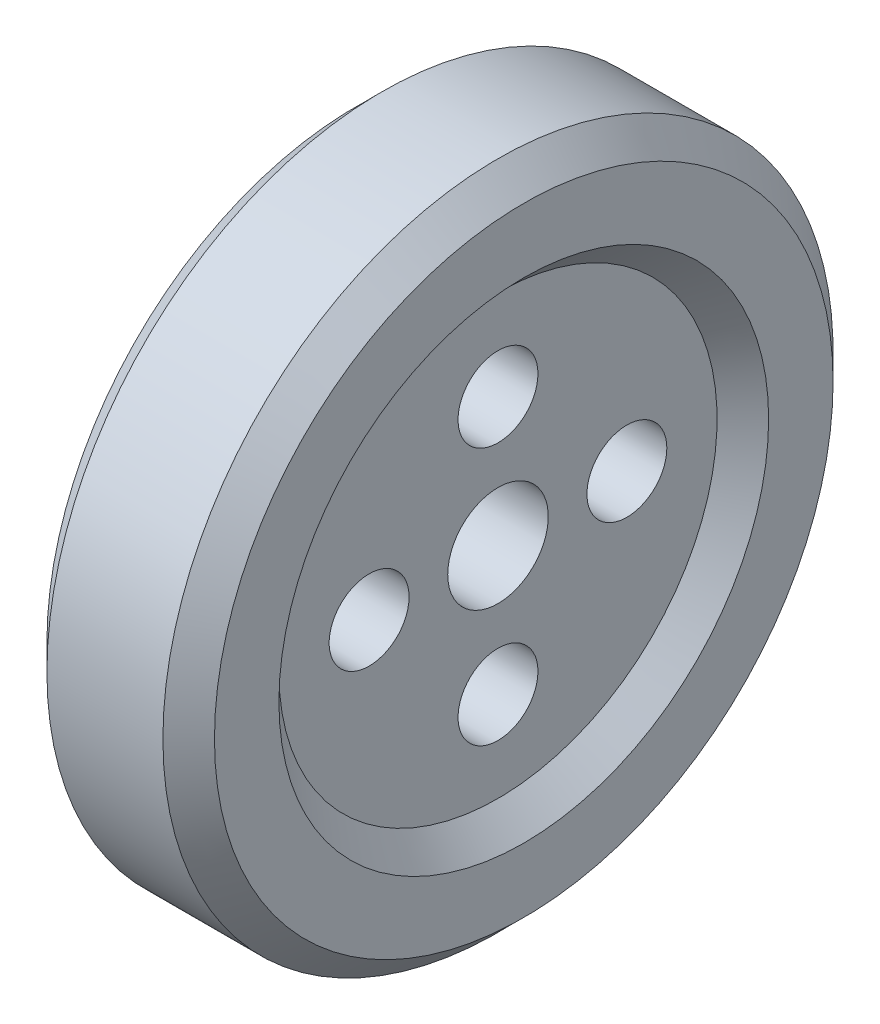
ISO-10303-21;
HEADER;
FILE_DESCRIPTION(('STEP AP214'),'2;1');
FILE_NAME('part.step','',(''),(''),'','','');
FILE_SCHEMA(('AUTOMOTIVE_DESIGN { 1 0 10303 214 1 1 1 1 }'));
ENDSEC;
DATA;
#1=APPLICATION_CONTEXT('core data for automotive mechanical design processes');
#2=APPLICATION_PROTOCOL_DEFINITION('international standard','automotive_design',2000,#1);
#3=PRODUCT_CONTEXT('',#1,'mechanical');
#4=PRODUCT('Part','Part','',(#3));
#5=PRODUCT_RELATED_PRODUCT_CATEGORY('part','',(#4));
#6=PRODUCT_DEFINITION_FORMATION('','',#4);
#7=PRODUCT_DEFINITION_CONTEXT('part definition',#1,'design');
#8=PRODUCT_DEFINITION('design','',#6,#7);
#9=PRODUCT_DEFINITION_SHAPE('','',#8);
#10=(LENGTH_UNIT() NAMED_UNIT(*) SI_UNIT(.MILLI.,.METRE.));
#11=(NAMED_UNIT(*) PLANE_ANGLE_UNIT() SI_UNIT($,.RADIAN.));
#12=(NAMED_UNIT(*) SI_UNIT($,.STERADIAN.) SOLID_ANGLE_UNIT());
#13=UNCERTAINTY_MEASURE_WITH_UNIT(LENGTH_MEASURE(1.E-05),#10,'distance_accuracy_value','');
#14=(GEOMETRIC_REPRESENTATION_CONTEXT(3) GLOBAL_UNCERTAINTY_ASSIGNED_CONTEXT((#13)) GLOBAL_UNIT_ASSIGNED_CONTEXT((#10,
#11,#12)) REPRESENTATION_CONTEXT('',''));
#15=CARTESIAN_POINT('',(0.,0.,0.));
#16=DIRECTION('',(0.,0.,1.));
#17=DIRECTION('',(1.,0.,0.));
#18=AXIS2_PLACEMENT_3D('',#15,#16,#17);
#19=CARTESIAN_POINT('',(-186.115918114073,0.,0.));
#20=DIRECTION('',(-1.,0.,0.));
#21=DIRECTION('',(0.,0.,1.));
#22=AXIS2_PLACEMENT_3D('',#19,#20,#21);
#23=CYLINDRICAL_SURFACE('',#22,260.);
#24=CARTESIAN_POINT('',(-45.,0.,0.));
#25=DIRECTION('',(-1.,0.,0.));
#26=DIRECTION('',(0.,0.,1.));
#27=AXIS2_PLACEMENT_3D('',#24,#25,#26);
#28=CIRCLE('',#27,260.);
#29=CARTESIAN_POINT('',(-45.,0.,260.));
#30=VERTEX_POINT('',#29);
#31=EDGE_CURVE('E10',#30,#30,#28,.T.);
#32=ORIENTED_EDGE('',*,*,#31,.F.);
#33=EDGE_LOOP('',(#32));
#34=FACE_BOUND('',#33,.T.);
#35=CARTESIAN_POINT('',(44.9999999999999,0.,0.));
#36=DIRECTION('',(-1.,0.,0.));
#37=DIRECTION('',(0.,0.,1.));
#38=AXIS2_PLACEMENT_3D('',#35,#36,#37);
#39=CIRCLE('',#38,260.);
#40=CARTESIAN_POINT('',(44.9999999999999,0.,260.));
#41=VERTEX_POINT('',#40);
#42=EDGE_CURVE('E72',#41,#41,#39,.T.);
#43=ORIENTED_EDGE('',*,*,#42,.T.);
#44=EDGE_LOOP('',(#43));
#45=FACE_BOUND('',#44,.T.);
#46=ADVANCED_FACE('F40',(#34,#45),#23,.T.);
#47=CARTESIAN_POINT('',(-45.,0.,0.));
#48=DIRECTION('',(1.,0.,0.));
#49=DIRECTION('',(0.,0.,-1.));
#50=AXIS2_PLACEMENT_3D('',#47,#48,#49);
#51=CONICAL_SURFACE('',#50,260.,0.785398163397452);
#52=CARTESIAN_POINT('',(-64.9999999999999,0.,0.));
#53=DIRECTION('',(-1.,0.,0.));
#54=DIRECTION('',(0.,0.,1.));
#55=AXIS2_PLACEMENT_3D('',#52,#53,#54);
#56=CIRCLE('',#55,240.);
#57=CARTESIAN_POINT('',(-64.9999999999999,0.,240.));
#58=VERTEX_POINT('',#57);
#59=EDGE_CURVE('E43',#58,#58,#56,.T.);
#60=ORIENTED_EDGE('',*,*,#59,.F.);
#61=EDGE_LOOP('',(#60));
#62=FACE_BOUND('',#61,.T.);
#63=ORIENTED_EDGE('',*,*,#31,.T.);
#64=EDGE_LOOP('',(#63));
#65=FACE_BOUND('',#64,.T.);
#66=ADVANCED_FACE('F136',(#62,#65),#51,.T.);
#67=CARTESIAN_POINT('',(-64.9999999999999,240.,0.));
#68=DIRECTION('',(1.,0.,0.));
#69=DIRECTION('',(0.,0.,-1.));
#70=AXIS2_PLACEMENT_3D('',#67,#68,#69);
#71=PLANE('',#70);
#72=CARTESIAN_POINT('',(-65.,0.,0.));
#73=DIRECTION('',(-1.,0.,0.));
#74=DIRECTION('',(0.,0.,1.));
#75=AXIS2_PLACEMENT_3D('',#72,#73,#74);
#76=CIRCLE('',#75,190.);
#77=CARTESIAN_POINT('',(-65.,0.,190.));
#78=VERTEX_POINT('',#77);
#79=EDGE_CURVE('E50',#78,#78,#76,.T.);
#80=ORIENTED_EDGE('',*,*,#79,.F.);
#81=EDGE_LOOP('',(#80));
#82=FACE_BOUND('',#81,.T.);
#83=ORIENTED_EDGE('',*,*,#59,.T.);
#84=EDGE_LOOP('',(#83));
#85=FACE_BOUND('',#84,.T.);
#86=ADVANCED_FACE('F135',(#82,#85),#71,.F.);
#87=CARTESIAN_POINT('',(-65.,0.,0.));
#88=DIRECTION('',(-1.,0.,0.));
#89=DIRECTION('',(0.,0.,1.));
#90=AXIS2_PLACEMENT_3D('',#87,#88,#89);
#91=CONICAL_SURFACE('',#90,190.,0.785398163397448);
#92=CARTESIAN_POINT('',(-45.,0.,0.));
#93=DIRECTION('',(-1.,0.,0.));
#94=DIRECTION('',(0.,0.,1.));
#95=AXIS2_PLACEMENT_3D('',#92,#93,#94);
#96=CIRCLE('',#95,170.);
#97=CARTESIAN_POINT('',(-45.,0.,170.));
#98=VERTEX_POINT('',#97);
#99=EDGE_CURVE('E51',#98,#98,#96,.T.);
#100=ORIENTED_EDGE('',*,*,#99,.F.);
#101=EDGE_LOOP('',(#100));
#102=FACE_BOUND('',#101,.T.);
#103=ORIENTED_EDGE('',*,*,#79,.T.);
#104=EDGE_LOOP('',(#103));
#105=FACE_BOUND('',#104,.T.);
#106=ADVANCED_FACE('F127',(#102,#105),#91,.F.);
#107=CARTESIAN_POINT('',(-45.,170.,0.));
#108=DIRECTION('',(1.,0.,0.));
#109=DIRECTION('',(0.,0.,-1.));
#110=AXIS2_PLACEMENT_3D('',#107,#108,#109);
#111=PLANE('',#110);
#112=CARTESIAN_POINT('',(-45.,100.,0.));
#113=DIRECTION('',(1.,0.,0.));
#114=DIRECTION('',(0.,0.,-1.));
#115=AXIS2_PLACEMENT_3D('',#112,#113,#114);
#116=CIRCLE('',#115,31.);
#117=CARTESIAN_POINT('',(-45.,100.,-31.));
#118=VERTEX_POINT('',#117);
#119=EDGE_CURVE('E74',#118,#118,#116,.F.);
#120=ORIENTED_EDGE('',*,*,#119,.F.);
#121=EDGE_LOOP('',(#120));
#122=FACE_BOUND('',#121,.T.);
#123=CARTESIAN_POINT('',(-45.,0.,-100.));
#124=DIRECTION('',(1.,0.,0.));
#125=DIRECTION('',(0.,0.,-1.));
#126=AXIS2_PLACEMENT_3D('',#123,#124,#125);
#127=CIRCLE('',#126,31.0000000000003);
#128=CARTESIAN_POINT('',(-45.,0.,-131.));
#129=VERTEX_POINT('',#128);
#130=EDGE_CURVE('E86',#129,#129,#127,.F.);
#131=ORIENTED_EDGE('',*,*,#130,.F.);
#132=EDGE_LOOP('',(#131));
#133=FACE_BOUND('',#132,.T.);
#134=CARTESIAN_POINT('',(-45.,-100.,0.));
#135=DIRECTION('',(1.,0.,0.));
#136=DIRECTION('',(0.,0.,-1.));
#137=AXIS2_PLACEMENT_3D('',#134,#135,#136);
#138=CIRCLE('',#137,31.0000000000007);
#139=CARTESIAN_POINT('',(-45.,-100.,-31.0000000000006));
#140=VERTEX_POINT('',#139);
#141=EDGE_CURVE('E85',#140,#140,#138,.F.);
#142=ORIENTED_EDGE('',*,*,#141,.F.);
#143=EDGE_LOOP('',(#142));
#144=FACE_BOUND('',#143,.T.);
#145=CARTESIAN_POINT('',(-45.,0.,100.));
#146=DIRECTION('',(1.,0.,0.));
#147=DIRECTION('',(0.,0.,-1.));
#148=AXIS2_PLACEMENT_3D('',#145,#146,#147);
#149=CIRCLE('',#148,31.000000000001);
#150=CARTESIAN_POINT('',(-45.,0.,68.999999999999));
#151=VERTEX_POINT('',#150);
#152=EDGE_CURVE('E73',#151,#151,#149,.F.);
#153=ORIENTED_EDGE('',*,*,#152,.F.);
#154=EDGE_LOOP('',(#153));
#155=FACE_BOUND('',#154,.T.);
#156=CARTESIAN_POINT('',(-45.,0.,0.));
#157=DIRECTION('',(-1.,0.,0.));
#158=DIRECTION('',(0.,0.,1.));
#159=AXIS2_PLACEMENT_3D('',#156,#157,#158);
#160=CIRCLE('',#159,39.);
#161=CARTESIAN_POINT('',(-45.,0.,39.));
#162=VERTEX_POINT('',#161);
#163=EDGE_CURVE('E57',#162,#162,#160,.T.);
#164=ORIENTED_EDGE('',*,*,#163,.F.);
#165=EDGE_LOOP('',(#164));
#166=FACE_BOUND('',#165,.T.);
#167=ORIENTED_EDGE('',*,*,#99,.T.);
#168=EDGE_LOOP('',(#167));
#169=FACE_BOUND('',#168,.T.);
#170=ADVANCED_FACE('F118',(#122,#133,#144,#155,#166,#169),#111,.F.);
#171=CARTESIAN_POINT('',(-186.115918114073,0.,0.));
#172=DIRECTION('',(-1.,0.,0.));
#173=DIRECTION('',(0.,0.,1.));
#174=AXIS2_PLACEMENT_3D('',#171,#172,#173);
#175=CYLINDRICAL_SURFACE('',#174,39.);
#176=CARTESIAN_POINT('',(45.,0.,0.));
#177=DIRECTION('',(-1.,0.,0.));
#178=DIRECTION('',(0.,0.,1.));
#179=AXIS2_PLACEMENT_3D('',#176,#177,#178);
#180=CIRCLE('',#179,39.);
#181=CARTESIAN_POINT('',(45.,0.,39.));
#182=VERTEX_POINT('',#181);
#183=EDGE_CURVE('E56',#182,#182,#180,.T.);
#184=ORIENTED_EDGE('',*,*,#183,.F.);
#185=EDGE_LOOP('',(#184));
#186=FACE_BOUND('',#185,.T.);
#187=ORIENTED_EDGE('',*,*,#163,.T.);
#188=EDGE_LOOP('',(#187));
#189=FACE_BOUND('',#188,.T.);
#190=ADVANCED_FACE('F106',(#186,#189),#175,.F.);
#191=CARTESIAN_POINT('',(45.,170.,0.));
#192=DIRECTION('',(-1.,0.,0.));
#193=DIRECTION('',(0.,0.,1.));
#194=AXIS2_PLACEMENT_3D('',#191,#192,#193);
#195=PLANE('',#194);
#196=CARTESIAN_POINT('',(45.,100.,0.));
#197=DIRECTION('',(1.,0.,0.));
#198=DIRECTION('',(0.,0.,-1.));
#199=AXIS2_PLACEMENT_3D('',#196,#197,#198);
#200=CIRCLE('',#199,31.);
#201=CARTESIAN_POINT('',(45.,100.,-31.));
#202=VERTEX_POINT('',#201);
#203=EDGE_CURVE('E93',#202,#202,#200,.T.);
#204=ORIENTED_EDGE('',*,*,#203,.F.);
#205=EDGE_LOOP('',(#204));
#206=FACE_BOUND('',#205,.T.);
#207=CARTESIAN_POINT('',(45.,0.,-100.));
#208=DIRECTION('',(1.,0.,0.));
#209=DIRECTION('',(0.,0.,-1.));
#210=AXIS2_PLACEMENT_3D('',#207,#208,#209);
#211=CIRCLE('',#210,31.0000000000003);
#212=CARTESIAN_POINT('',(45.,0.,-131.));
#213=VERTEX_POINT('',#212);
#214=EDGE_CURVE('E84',#213,#213,#211,.T.);
#215=ORIENTED_EDGE('',*,*,#214,.F.);
#216=EDGE_LOOP('',(#215));
#217=FACE_BOUND('',#216,.T.);
#218=CARTESIAN_POINT('',(45.,-100.,0.));
#219=DIRECTION('',(1.,0.,0.));
#220=DIRECTION('',(0.,0.,-1.));
#221=AXIS2_PLACEMENT_3D('',#218,#219,#220);
#222=CIRCLE('',#221,31.0000000000007);
#223=CARTESIAN_POINT('',(45.,-100.,-31.0000000000006));
#224=VERTEX_POINT('',#223);
#225=EDGE_CURVE('E80',#224,#224,#222,.T.);
#226=ORIENTED_EDGE('',*,*,#225,.F.);
#227=EDGE_LOOP('',(#226));
#228=FACE_BOUND('',#227,.T.);
#229=CARTESIAN_POINT('',(45.,0.,100.));
#230=DIRECTION('',(1.,0.,0.));
#231=DIRECTION('',(0.,0.,-1.));
#232=AXIS2_PLACEMENT_3D('',#229,#230,#231);
#233=CIRCLE('',#232,31.000000000001);
#234=CARTESIAN_POINT('',(45.,0.,68.999999999999));
#235=VERTEX_POINT('',#234);
#236=EDGE_CURVE('E76',#235,#235,#233,.T.);
#237=ORIENTED_EDGE('',*,*,#236,.F.);
#238=EDGE_LOOP('',(#237));
#239=FACE_BOUND('',#238,.T.);
#240=CARTESIAN_POINT('',(45.,0.,0.));
#241=DIRECTION('',(-1.,0.,0.));
#242=DIRECTION('',(0.,0.,1.));
#243=AXIS2_PLACEMENT_3D('',#240,#241,#242);
#244=CIRCLE('',#243,170.);
#245=CARTESIAN_POINT('',(45.,0.,170.));
#246=VERTEX_POINT('',#245);
#247=EDGE_CURVE('E64',#246,#246,#244,.T.);
#248=ORIENTED_EDGE('',*,*,#247,.F.);
#249=EDGE_LOOP('',(#248));
#250=FACE_BOUND('',#249,.T.);
#251=ORIENTED_EDGE('',*,*,#183,.T.);
#252=EDGE_LOOP('',(#251));
#253=FACE_BOUND('',#252,.T.);
#254=ADVANCED_FACE('F105',(#206,#217,#228,#239,#250,#253),#195,.F.);
#255=CARTESIAN_POINT('',(45.,0.,0.));
#256=DIRECTION('',(1.,0.,0.));
#257=DIRECTION('',(0.,0.,-1.));
#258=AXIS2_PLACEMENT_3D('',#255,#256,#257);
#259=CONICAL_SURFACE('',#258,170.,0.785398163397447);
#260=CARTESIAN_POINT('',(65.,0.,0.));
#261=DIRECTION('',(-1.,0.,0.));
#262=DIRECTION('',(0.,0.,1.));
#263=AXIS2_PLACEMENT_3D('',#260,#261,#262);
#264=CIRCLE('',#263,190.);
#265=CARTESIAN_POINT('',(65.,0.,190.));
#266=VERTEX_POINT('',#265);
#267=EDGE_CURVE('E63',#266,#266,#264,.T.);
#268=ORIENTED_EDGE('',*,*,#267,.F.);
#269=EDGE_LOOP('',(#268));
#270=FACE_BOUND('',#269,.T.);
#271=ORIENTED_EDGE('',*,*,#247,.T.);
#272=EDGE_LOOP('',(#271));
#273=FACE_BOUND('',#272,.T.);
#274=ADVANCED_FACE('F104',(#270,#273),#259,.F.);
#275=CARTESIAN_POINT('',(65.,240.,0.));
#276=DIRECTION('',(-1.,0.,0.));
#277=DIRECTION('',(0.,0.,1.));
#278=AXIS2_PLACEMENT_3D('',#275,#276,#277);
#279=PLANE('',#278);
#280=CARTESIAN_POINT('',(65.,0.,0.));
#281=DIRECTION('',(-1.,0.,0.));
#282=DIRECTION('',(0.,0.,1.));
#283=AXIS2_PLACEMENT_3D('',#280,#281,#282);
#284=CIRCLE('',#283,240.);
#285=CARTESIAN_POINT('',(65.,0.,240.));
#286=VERTEX_POINT('',#285);
#287=EDGE_CURVE('E66',#286,#286,#284,.T.);
#288=ORIENTED_EDGE('',*,*,#287,.F.);
#289=EDGE_LOOP('',(#288));
#290=FACE_BOUND('',#289,.T.);
#291=ORIENTED_EDGE('',*,*,#267,.T.);
#292=EDGE_LOOP('',(#291));
#293=FACE_BOUND('',#292,.T.);
#294=ADVANCED_FACE('F154',(#290,#293),#279,.F.);
#295=CARTESIAN_POINT('',(65.,0.,0.));
#296=DIRECTION('',(-1.,0.,0.));
#297=DIRECTION('',(0.,0.,1.));
#298=AXIS2_PLACEMENT_3D('',#295,#296,#297);
#299=CONICAL_SURFACE('',#298,240.,0.785398163397446);
#300=ORIENTED_EDGE('',*,*,#42,.F.);
#301=EDGE_LOOP('',(#300));
#302=FACE_BOUND('',#301,.T.);
#303=ORIENTED_EDGE('',*,*,#287,.T.);
#304=EDGE_LOOP('',(#303));
#305=FACE_BOUND('',#304,.T.);
#306=ADVANCED_FACE('F151',(#302,#305),#299,.T.);
#307=CARTESIAN_POINT('',(-65.001,0.,100.));
#308=DIRECTION('',(1.,0.,0.));
#309=DIRECTION('',(0.,0.,-1.));
#310=AXIS2_PLACEMENT_3D('',#307,#308,#309);
#311=CYLINDRICAL_SURFACE('',#310,31.000000000001);
#312=ORIENTED_EDGE('',*,*,#236,.T.);
#313=EDGE_LOOP('',(#312));
#314=FACE_BOUND('',#313,.T.);
#315=ORIENTED_EDGE('',*,*,#152,.T.);
#316=EDGE_LOOP('',(#315));
#317=FACE_BOUND('',#316,.T.);
#318=ADVANCED_FACE('F152',(#314,#317),#311,.F.);
#319=CARTESIAN_POINT('',(-65.001,-100.,0.));
#320=DIRECTION('',(1.,0.,0.));
#321=DIRECTION('',(0.,0.,-1.));
#322=AXIS2_PLACEMENT_3D('',#319,#320,#321);
#323=CYLINDRICAL_SURFACE('',#322,31.0000000000007);
#324=ORIENTED_EDGE('',*,*,#225,.T.);
#325=EDGE_LOOP('',(#324));
#326=FACE_BOUND('',#325,.T.);
#327=ORIENTED_EDGE('',*,*,#141,.T.);
#328=EDGE_LOOP('',(#327));
#329=FACE_BOUND('',#328,.T.);
#330=ADVANCED_FACE('F174',(#326,#329),#323,.F.);
#331=CARTESIAN_POINT('',(-65.001,0.,-100.));
#332=DIRECTION('',(1.,0.,0.));
#333=DIRECTION('',(0.,0.,-1.));
#334=AXIS2_PLACEMENT_3D('',#331,#332,#333);
#335=CYLINDRICAL_SURFACE('',#334,31.0000000000003);
#336=ORIENTED_EDGE('',*,*,#214,.T.);
#337=EDGE_LOOP('',(#336));
#338=FACE_BOUND('',#337,.T.);
#339=ORIENTED_EDGE('',*,*,#130,.T.);
#340=EDGE_LOOP('',(#339));
#341=FACE_BOUND('',#340,.T.);
#342=ADVANCED_FACE('F178',(#338,#341),#335,.F.);
#343=CARTESIAN_POINT('',(-65.001,100.,0.));
#344=DIRECTION('',(1.,0.,0.));
#345=DIRECTION('',(0.,0.,-1.));
#346=AXIS2_PLACEMENT_3D('',#343,#344,#345);
#347=CYLINDRICAL_SURFACE('',#346,31.);
#348=ORIENTED_EDGE('',*,*,#203,.T.);
#349=EDGE_LOOP('',(#348));
#350=FACE_BOUND('',#349,.T.);
#351=ORIENTED_EDGE('',*,*,#119,.T.);
#352=EDGE_LOOP('',(#351));
#353=FACE_BOUND('',#352,.T.);
#354=ADVANCED_FACE('F97',(#350,#353),#347,.F.);
#355=CLOSED_SHELL('',(#46,#66,#86,#106,#170,#190,#254,#274,#294,#306,#318,#330,#342,#354));
#356=MANIFOLD_SOLID_BREP('B2',#355);
#357=ADVANCED_BREP_SHAPE_REPRESENTATION('',(#18,#356),#14);
#358=SHAPE_DEFINITION_REPRESENTATION(#9,#357);
ENDSEC;
END-ISO-10303-21;
